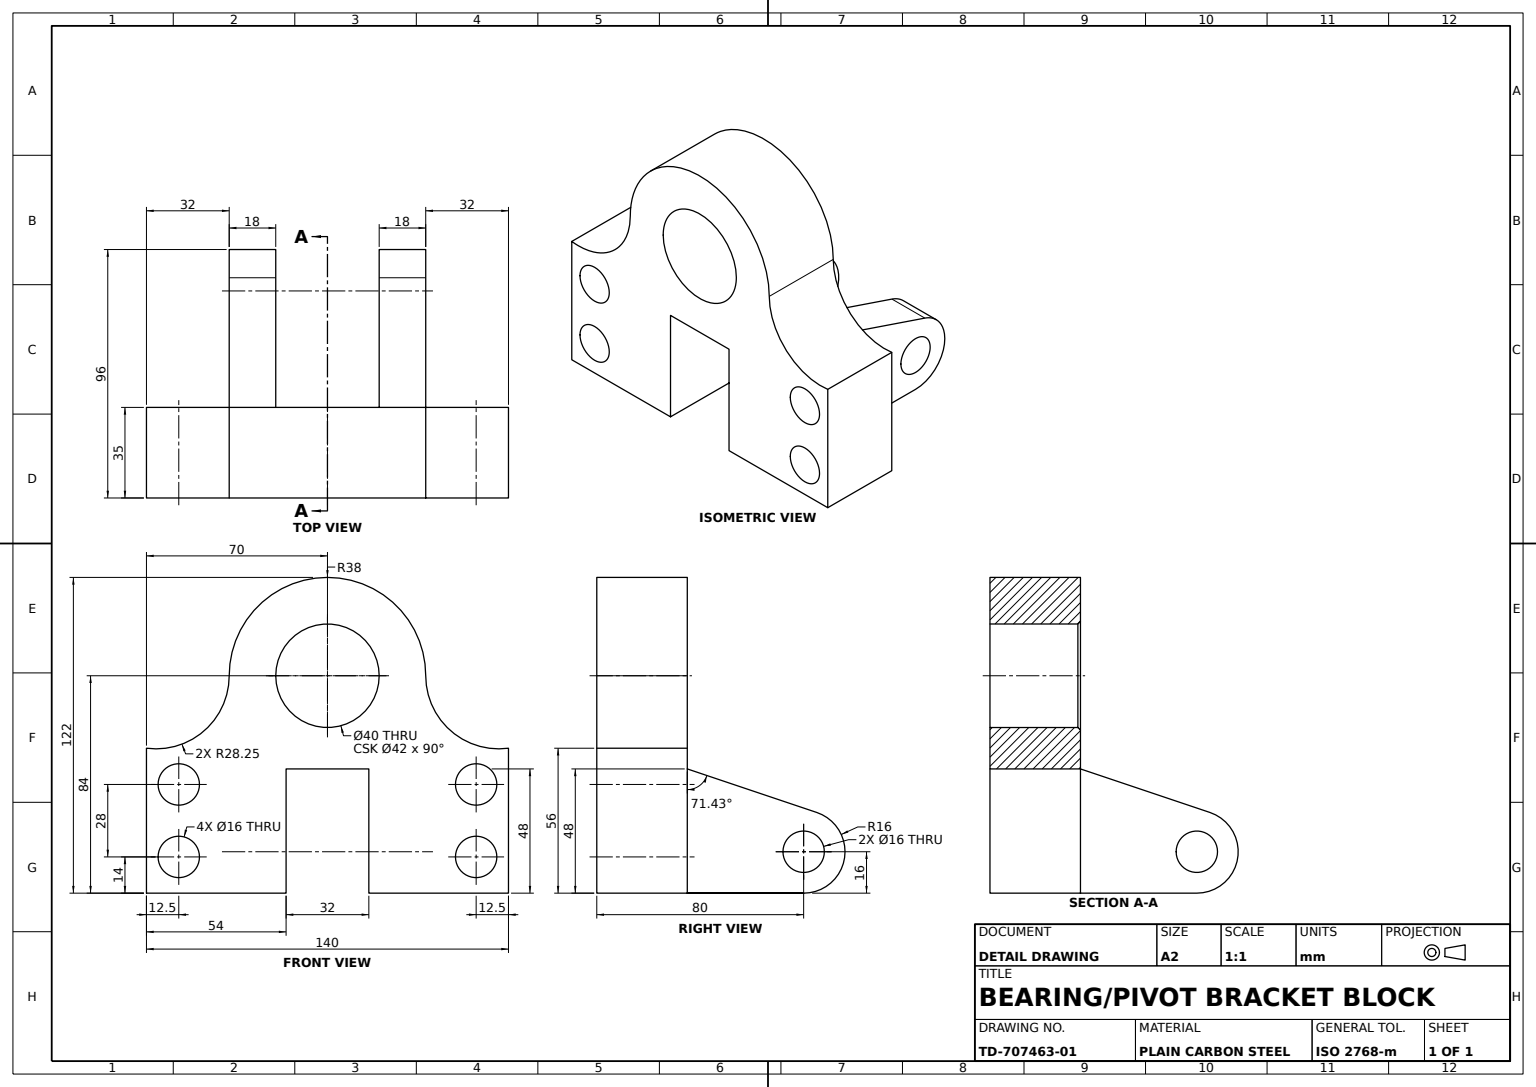
from build123d import *

# Parameters (mm, degrees)
BASE_BLOCK_DEPTH         = 35
BORE_PROFILE_R           = 20
BORE_40_DEPTH            = 35
MOUNTING_HOLES_PROFILE_R = 8
MOUNTING_HOLES_4X_DEPTH  = 35
SIDE_ARM_PROFILE_R       = 8
SIDE_ARM_DEPTH           = 18
LUG_START                = 18
LUG_BOSS_PROFILE_R       = 8
LUG_BOSS_DEPTH           = 18
RELIEF_CUT_PROFILE_W     = 32
RELIEF_CUT_PROFILE_H     = 48
RELIEF_CUT_DEPTH         = 35
BORE_CHAMFER_1MM_SIZE    = 1


with BuildPart() as part:
    # Base Block Profile → Base Block (new body)
    with BuildSketch(Plane.XY):
        with BuildLine():
            Line((-70, -28), (-70, -84))
            Line((-70, -84), (70, -84))
            Line((70, -84), (70, -28))
            ThreePointArc((70, -28), (47.647244828, -21.260291625), (38, 0))
            ThreePointArc((38, 0), (0, 38), (-38, 0))
            ThreePointArc((-38, 0), (-47.647244828, -21.260291625), (-70, -28))
        make_face()
    extrude(amount=BASE_BLOCK_DEPTH)

    # Bore Profile → Bore Ø40 (cut)
    with BuildSketch(Plane.XY.offset(35)):
        Circle(BORE_PROFILE_R)
    extrude(amount=-BORE_40_DEPTH, mode=Mode.SUBTRACT)

    # Mounting Holes Profile → Mounting Holes 4x (cut)
    with BuildSketch(Plane.XY.offset(35)):
        with Locations((-57.5, -42)):
            Circle(MOUNTING_HOLES_PROFILE_R)
        with Locations((-57.5, -70)):
            Circle(MOUNTING_HOLES_PROFILE_R)
        with Locations((57.5, -42)):
            Circle(MOUNTING_HOLES_PROFILE_R)
        with Locations((57.5, -70)):
            Circle(MOUNTING_HOLES_PROFILE_R)
    extrude(amount=-MOUNTING_HOLES_4X_DEPTH, mode=Mode.SUBTRACT)

    # Side Arm Profile → Side Arm (add)
    with BuildSketch(Plane(origin=(38, 0, 0), x_dir=(0, 0, -1), z_dir=(1, 0, 0))):
        with BuildLine():
            Line((0, -84), (0, -36))
            Line((0, -36), (50.096296037, -52.833333698))
            ThreePointArc((50.096296037, -52.833333698), (60.790292284, -70.581989463), (45, -84))
            Line((45, -84), (0, -84))
        make_face()
        with Locations((45, -68)):
            Circle(SIDE_ARM_PROFILE_R, mode=Mode.SUBTRACT)
    extrude(amount=-SIDE_ARM_DEPTH)

    # Lug Boss Profile → Lug Boss (add)
    with BuildSketch(Plane(origin=(-38, 0, 0), x_dir=(0, 0, -1), z_dir=(1, 0, 0)).offset(LUG_START)):
        with BuildLine():
            Line((0, -36), (0, -84))
            Line((0, -84), (45, -84))
            ThreePointArc((45, -84), (60.790292284, -70.581989463), (50.096296037, -52.833333698))
            Line((50.096296037, -52.833333698), (0, -36))
        make_face()
        with Locations((45, -68)):
            Circle(LUG_BOSS_PROFILE_R, mode=Mode.SUBTRACT)
    extrude(amount=-LUG_BOSS_DEPTH)

    # Relief Cut Profile → Relief Cut (cut)
    with BuildSketch(Plane(origin=(0, 0, 0), x_dir=(-1, 0, 0), z_dir=(0, 0, -1))):
        with Locations((0, -60)):
            Rectangle(RELIEF_CUT_PROFILE_W, RELIEF_CUT_PROFILE_H)
    extrude(amount=-RELIEF_CUT_DEPTH, mode=Mode.SUBTRACT)

    # Bore Chamfer 1mm
    bore_chamfer_1mm_edges = [part.edges().sort_by_distance(p)[0] for p in [
        (-20, 0, 0),
    ]]
    chamfer(bore_chamfer_1mm_edges, length=BORE_CHAMFER_1MM_SIZE)


solid = part.part
